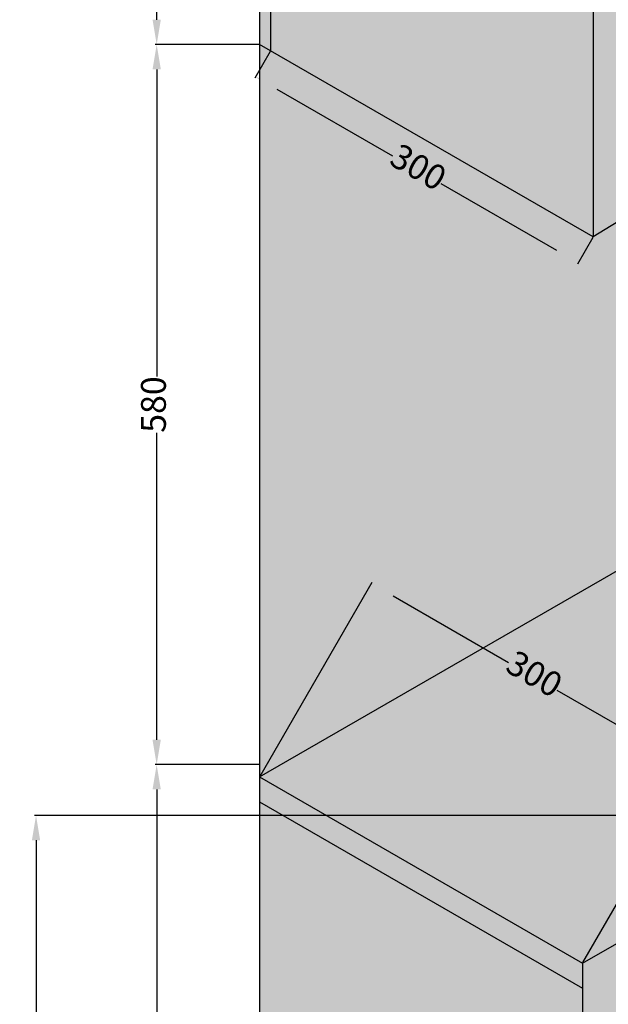
# Model space of a CAD drawing. Units: millimetres. Extents: x 78378 to 86415, y 148682 to 152721.
# Tile 2 of 18: x 78378 to 78851, y 149702 to 150495. Entities that reach past the tile are written whole.
import ezdxf

# ---------------------------------------------------------------- set-up
doc = ezdxf.new("R2010")
doc.units = ezdxf.units.MM
for name, color, linetype, lineweight in [('A-ANNO-DIMS', 2, 'Continuous', 18), ('A-FURN', 4, 'Continuous', 25), ('A-FURN-PATT', 32, 'Continuous', 13)]:
    doc.layers.add(name, color=color, linetype=linetype, lineweight=lineweight)
doc.styles.get("Standard").update_dxf_attribs({"font": 'arial.ttf'})
doc.dimstyles.new('ISO-25', dxfattribs={"dimtxt": 20, "dimasz": 20, "dimexe": 1.25, "dimexo": 0.625, "dimtad": 0, "dimdec": 1, "dimtxsty": 'Standard', "dimcen": 2.5, "dimadec": 0, "dimazin": 0, "dimtfac": 1, "dimtdec": 1, "dimtmove": 0, "dimatfit": 3, "dimfxl": 1, "dimarcsym": 0})

# ---------------------------------------------------------------- blocks, each defined once
blk = doc.blocks.new('*D4')
at = {"layer": 'A-ANNO-DIMS', "color": 0, "lineweight": -2, "transparency": 16777216}
for p, q in [((78570.23, 151205.01), (78486.72, 151205.01)), ((78487.97, 151185.01), (78487.97, 150862.61)), ((78487.97, 150495.01), (78487.97, 150817.4)), ((78570.23, 150475.01), (78486.72, 150475.01))]:
    blk.add_line(p, q, dxfattribs=at)
at = {"layer": 'A-ANNO-DIMS', "color": 0, "transparency": 16777216}
for points in [[(78484.64, 151185.01), (78491.3, 151185.01), (78487.97, 151205.01)], [(78484.64, 150495.01), (78491.3, 150495.01), (78487.97, 150475.01)]]:
    blk.add_solid(points, dxfattribs=at)
at = {"layer": 'Defpoints', "color": 0, "transparency": 16777216}
for p in [(78570.86, 151205.01), (78487.97, 150475.01), (78570.86, 150475.01)]:
    blk.add_point(p, dxfattribs=at)
at = {"layer": 'A-ANNO-DIMS', "color": 0, "transparency": 16777216, "insert": (78487.97, 150840.01), "char_height": 20, "attachment_point": 5, "rotation": 90}
blk.add_mtext('730', dxfattribs=at)
blk = doc.blocks.new('*D5')
at = {"layer": 'A-ANNO-DIMS', "color": 0, "lineweight": -2, "transparency": 16777216}
for p, q in [((78570.23, 150475.01), (78486.72, 150475.01)), ((78487.97, 150455.01), (78487.97, 150207.69)), ((78487.97, 149915.01), (78487.97, 150162.32)), ((78570.23, 149895.01), (78486.72, 149895.01))]:
    blk.add_line(p, q, dxfattribs=at)
at = {"layer": 'A-ANNO-DIMS', "color": 0, "transparency": 16777216}
for points in [[(78484.64, 150455.01), (78491.3, 150455.01), (78487.97, 150475.01)], [(78484.64, 149915.01), (78491.3, 149915.01), (78487.97, 149895.01)]]:
    blk.add_solid(points, dxfattribs=at)
at = {"layer": 'Defpoints', "color": 0, "transparency": 16777216}
for p in [(78570.86, 150475.01), (78487.97, 149895.01), (78570.86, 149895.01)]:
    blk.add_point(p, dxfattribs=at)
at = {"layer": 'A-ANNO-DIMS', "color": 0, "transparency": 16777216, "insert": (78487.97, 150185.01), "char_height": 20, "attachment_point": 5, "rotation": 90}
blk.add_mtext('580', dxfattribs=at)
blk = doc.blocks.new('*D6')
at = {"layer": 'A-ANNO-DIMS', "color": 0, "lineweight": -2, "transparency": 16777216}
for p, q in [((78570.23, 149895.01), (78486.72, 149895.01)), ((78487.97, 149875.01), (78487.97, 149487.71)), ((78487.97, 149055.01), (78487.97, 149442.31)), ((78570.23, 149035.01), (78486.72, 149035.01))]:
    blk.add_line(p, q, dxfattribs=at)
at = {"layer": 'A-ANNO-DIMS', "color": 0, "transparency": 16777216}
for points in [[(78484.64, 149875.01), (78491.3, 149875.01), (78487.97, 149895.01)], [(78484.64, 149055.01), (78491.3, 149055.01), (78487.97, 149035.01)]]:
    blk.add_solid(points, dxfattribs=at)
at = {"layer": 'Defpoints', "color": 0, "transparency": 16777216}
for p in [(78570.86, 149895.01), (78487.97, 149035.01), (78570.86, 149035.01)]:
    blk.add_point(p, dxfattribs=at)
at = {"layer": 'A-ANNO-DIMS', "color": 0, "transparency": 16777216, "insert": (78487.97, 149465.01), "char_height": 20, "attachment_point": 5, "rotation": 90}
blk.add_mtext('860', dxfattribs=at)
blk = doc.blocks.new('*D7')
at = {"layer": 'A-ANNO-DIMS', "color": 0, "lineweight": -2, "transparency": 16777216}
for p, q in [((78579.21, 150469.47), (78566.84, 150448.04)), ((78584.78, 150439.12), (78677.72, 150385.46)), ((78809.95, 150309.12), (78717, 150362.78)), ((78839.02, 150319.47), (78826.64, 150298.04))]:
    blk.add_line(p, q, dxfattribs=at)
at = {"layer": 'A-ANNO-DIMS', "color": 0, "transparency": 16777216}
for points in [[(78586.45, 150442.01), (78583.11, 150436.23), (78567.46, 150449.12)], [(78811.61, 150312.01), (78808.28, 150306.23), (78827.27, 150299.12)]]:
    blk.add_solid(points, dxfattribs=at)
at = {"layer": 'Defpoints', "color": 0, "transparency": 16777216}
for p in [(78579.52, 150470.01), (78567.46, 150449.12), (78839.33, 150320.01)]:
    blk.add_point(p, dxfattribs=at)
at = {"layer": 'A-ANNO-DIMS', "color": 0, "transparency": 16777216, "insert": (78697.36, 150374.12), "char_height": 20, "attachment_point": 5, "rotation": 330}
blk.add_mtext('300', dxfattribs=at)
blk = doc.blocks.new('*D19')
at = {"layer": 'A-ANNO-DIMS', "color": 0, "lineweight": -2, "transparency": 16777216}
for p, q in [((78571.17, 149885.55), (78661.48, 150041.97)), ((78678.18, 150030.89), (78771.12, 149977.23)), ((78903.35, 149900.89), (78810.4, 149954.55)), ((78830.98, 149735.55), (78921.29, 149891.97))]:
    blk.add_line(p, q, dxfattribs=at)
at = {"layer": 'A-ANNO-DIMS', "color": 0, "transparency": 16777216}
for points in [[(78679.85, 150033.78), (78676.51, 150028.01), (78660.86, 150040.89)], [(78905.01, 149903.78), (78901.68, 149898.01), (78920.67, 149890.89)]]:
    blk.add_solid(points, dxfattribs=at)
at = {"layer": 'Defpoints', "color": 0, "transparency": 16777216}
for p in [(78920.67, 149890.89), (78570.86, 149885.01), (78830.67, 149735.01)]:
    blk.add_point(p, dxfattribs=at)
at = {"layer": 'A-ANNO-DIMS', "color": 0, "transparency": 16777216, "insert": (78790.76, 149965.89), "char_height": 20, "attachment_point": 5, "rotation": 330}
blk.add_mtext('300', dxfattribs=at)
blk = doc.blocks.new('*D25')
at = {"layer": 'A-ANNO-DIMS', "color": 0, "lineweight": -2, "transparency": 16777216}
for p, q in [((79360.48, 149854.03), (78389.61, 149854.03)), ((78390.86, 149834.03), (78390.86, 149656.62)), ((78390.86, 149409.86), (78390.86, 149587.28)), ((79360.48, 149389.86), (78389.61, 149389.86))]:
    blk.add_line(p, q, dxfattribs=at)
at = {"layer": 'A-ANNO-DIMS', "color": 0, "transparency": 16777216}
for points in [[(78387.53, 149834.03), (78394.19, 149834.03), (78390.86, 149854.03)], [(78387.53, 149409.86), (78394.19, 149409.86), (78390.86, 149389.86)]]:
    blk.add_solid(points, dxfattribs=at)
at = {"layer": 'Defpoints', "color": 0, "transparency": 16777216}
for p in [(78390.86, 149854.03), (79361.1, 149854.03), (79361.1, 149389.86)]:
    blk.add_point(p, dxfattribs=at)
at = {"layer": 'A-ANNO-DIMS', "color": 0, "transparency": 16777216, "insert": (78390.86, 149621.95), "char_height": 20, "attachment_point": 5, "rotation": 90}
blk.add_mtext('464.2', dxfattribs=at)

msp = doc.modelspace()

# ---------------------------------------------------------------- hatches: boundary and pattern name
at = {"layer": 'A-FURN-PATT'}
h = msp.add_hatch(color=256, dxfattribs=at)
h.dxf.hatch_style = 1
h.paths.add_polyline_path([(78839.3276, 151040.0076), (78579.52, 151190.0076), (78579.52, 150470.0076), (78839.3276, 150320.0076)])
h.paths.add_polyline_path([(79073.1545, 150899.6469, 0.27777969), (79002.2645, 150996.3205, 0.79108393), (78917.9567, 150978.8719, 0.18044832), (78856.6481, 150853.0138), (78856.6481, 150350.6973), (79073.1545, 150484.318)])
h.paths.add_polyline_path([(79073.1545, 151175.0076), (78856.6481, 151050.0076), (78856.6481, 150853.0138, -0.18044832), (78917.9567, 150978.8719, -0.79108393), (79002.2645, 150996.3205, -0.27777969), (79073.1545, 150899.6469)])
h.paths.add_polyline_path([(79341.6224, 151350.0076), (79099.1352, 151490.0076), (78596.8405, 151200.0076), (78839.3276, 151060.0076)])
h.paths.add_polyline_path([(79904.5389, 151675.0076), (79662.0518, 151815.0076), (79099.1352, 151490.0076), (79341.6224, 151350.0076)])
h.paths.add_polyline_path([(80389.5131, 151955.0076), (80389.5131, 152235.0076), (79662.0518, 151815.0076), (79904.5389, 151675.0076)])
h.paths.add_polyline_path([(80389.5131, 151955.0076), (80164.3465, 151825.0076), (80164.3465, 151105.0076), (80614.6797, 151105.0076), (80614.6797, 151825.0076)])
edge = h.paths.add_edge_path(flags=16)
edge.add_spline(control_points=[(80216.308, 151728.251), (80227.1854, 151732.981), (80256.3301, 151745.6544), (80298.41, 151761.9595), (80340.2597, 151805.855), (80391.0771, 151782.0404), (80454.0396, 151805.7581), (80496.5007, 151742.4095), (80543.8218, 151733.4043), (80562.7182, 151729.8083)], knot_values=[0, 0, 0, 0, 35.54374676, 95.23575347, 136.36767513, 200.93298197, 236.72641081, 322.88993498, 380.17027367, 380.17027367, 380.17027367, 380.17027367], degree=3, periodic=0)
edge.add_line((80562.7182, 151729.8083), (80562.7182, 151165.0076))
edge.add_line((80562.7182, 151165.0076), (80216.308, 151165.0076))
edge.add_line((80216.308, 151165.0076), (80216.308, 151728.251))
h.paths.add_polyline_path([(80632.0002, 152095.0076), (80389.5131, 152235.0076), (80389.5131, 151955.0076), (80614.6797, 151825.0076), (80632.0002, 151815.0076)])
h.paths.add_polyline_path([(80867.7794, 151958.8805), (80632.0002, 152095.0076), (80632.0002, 151815.0076), (80632.0002, 151510.0076), (80867.7794, 151373.8805)])
h.paths.add_polyline_path([(80147.026, 151495.8203, 0.18918979), (80063.5671, 151597.7244, 0.78826136), (79979.2691, 151580.5832, 0.16072613), (79904.5389, 151413.5769), (79904.5389, 150955.0076), (80147.026, 151095.0076)])
h.paths.add_polyline_path([(80147.026, 151815.0076), (79904.5389, 151675.0076), (79904.5389, 151413.5769, -0.16072613), (79979.2691, 151580.5832, -0.78826136), (80063.5671, 151597.7244, -0.18918979), (80147.026, 151495.8203)])
h.paths.add_polyline_path([(79887.2184, 151645.0076), (79640.4011, 151502.5076), (79640.4011, 151262.3325, -0.16072613), (79715.1313, 151429.3387, -0.78826136), (79799.4294, 151446.48, -0.21290578), (79887.2184, 151328.7247)])
h.paths.add_polyline_path([(79799.4294, 151446.48, 0.78826136), (79715.1313, 151429.3387, 0.16072613), (79640.4011, 151262.3325), (79640.4011, 150822.5076), (79887.2184, 150965.0076), (79887.2184, 151328.7247, 0.21290578)])
h.paths.add_polyline_path([(79605.7601, 151482.5076), (79358.9429, 151340.0076), (79358.9429, 151100.0701, -0.16072613), (79433.6731, 151267.0764, -0.78826136), (79517.9711, 151284.2176, -0.21290578), (79605.7601, 151166.4623)])
h.paths.add_polyline_path([(79605.7601, 151166.4623, 0.21290578), (79517.9711, 151284.2176, 0.78826136), (79433.6731, 151267.0764, 0.16072613), (79358.9429, 151100.0701), (79358.9429, 150742.9831), (79419.0877, 150694.7323), (79605.7601, 150802.5076)])
edge = h.paths.add_edge_path(flags=0)
edge.add_spline(control_points=[(81152.4356, 151098.7676), (81105.7208, 151145.9466), (81038.6136, 151213.7208), (80882.3866, 151214.1938), (80797.4434, 151311.2997), (80711.8686, 151340.3754), (80681.7691, 151350.6023)], knot_values=[0, 0, 0, 0, 188.233441, 270.4032752, 445.45179201, 540.42858829, 540.42858829, 540.42858829, 540.42858829], degree=3, periodic=0)
edge.add_line((80683.4538, 151350.0269), (80683.4538, 151104.8792))
edge.add_line((80683.4538, 151104.8792), (81152.4356, 150851.399))
edge.add_line((81152.4356, 150851.399), (81152.4356, 151098.7676))
edge = h.paths.add_edge_path(flags=0)
edge.add_spline(control_points=[(80912.9018, 151027.1103), (80892.3742, 151034.1027), (80860.1663, 151045.0739), (80835.5097, 151068.1214), (80826.5679, 151076.4797)], knot_values=[0, 0, 0, 0, 63.98405104, 100.39142428, 100.39142428, 100.39142428, 100.39142428], degree=3, periodic=0)
edge.add_arc((80830.0414, 151081.2992), 5.9407, 100.9277276, 234.2187381, ccw=False)
edge.add_spline(control_points=[(80828.9152, 151087.1322), (80837.857, 151078.7739), (80862.5136, 151055.7263), (80894.7215, 151044.7552), (80915.2491, 151037.7628)], knot_values=[0, 0, 0, 0, 36.40737324, 100.39142428, 100.39142428, 100.39142428, 100.39142428], degree=3, periodic=0)
edge.add_arc((80914.7882, 151032.2795), 5.5026, -107.9540399, 85.195579, ccw=False)
h.paths.add_polyline_path([(81238.218, 151110.0076), (80632.0002, 151460.0076), (80632.0002, 151105.0076), (81238.218, 150755.0076)])
edge = h.paths.add_edge_path(flags=16)
edge.add_line((81152.4356, 150851.399), (80683.4538, 151104.8792))
edge.add_line((80683.4538, 151104.8792), (80683.4538, 151350.0279))
edge.add_spline(control_points=[(80681.7691, 151350.6023), (80711.8686, 151340.3754), (80797.4434, 151311.2997), (80882.3866, 151214.1938), (81038.6136, 151213.7208), (81105.7208, 151145.9466), (81152.4356, 151098.7676)], knot_values=[0, 0, 0, 0, 94.97679628, 270.02531309, 352.19514729, 540.42858829, 540.42858829, 540.42858829, 540.42858829], degree=3, periodic=0)
edge.add_line((81152.4356, 151098.7676), (81152.4356, 150851.399))
edge = h.paths.add_edge_path(flags=0)
edge.add_spline(control_points=[(80912.9018, 151027.1103), (80892.3742, 151034.1027), (80860.1663, 151045.0739), (80835.5097, 151068.1214), (80826.5679, 151076.4797)], knot_values=[0, 0, 0, 0, 63.98405104, 100.39142428, 100.39142428, 100.39142428, 100.39142428], degree=3, periodic=0)
edge.add_arc((80830.0414, 151081.2992), 5.9407, 100.9277276, 234.2187381, ccw=False)
edge.add_spline(control_points=[(80828.9152, 151087.1322), (80837.857, 151078.7739), (80862.5136, 151055.7263), (80894.7215, 151044.7552), (80915.2491, 151037.7628)], knot_values=[0, 0, 0, 0, 36.40737324, 100.39142428, 100.39142428, 100.39142428, 100.39142428], degree=3, periodic=0)
edge.add_arc((80914.7882, 151032.2795), 5.5026, -107.7417882, 85.195579, ccw=False)
h.paths.add_polyline_path([(81498.0256, 151255.0076), (81238.218, 151110.0076), (81238.218, 150755.0076), (81498.0256, 150905.0076)])
edge = h.paths.add_edge_path(flags=16)
edge.add_spline(control_points=[(81152.4356, 151098.7676), (81105.7208, 151145.9466), (81038.6136, 151213.7208), (80882.3866, 151214.1938), (80797.4434, 151311.2997), (80711.8686, 151340.3754), (80681.7691, 151350.6023)], knot_values=[0, 0, 0, 0, 188.233441, 270.4032752, 445.45179201, 540.42858829, 540.42858829, 540.42858829, 540.42858829], degree=3, periodic=0)
edge.add_line((80683.4538, 151350.0279), (80683.4538, 151104.8792))
edge.add_line((80683.4538, 151104.8792), (81152.4356, 150851.399))
edge.add_line((81152.4356, 150851.399), (81152.4356, 151098.7676))
h.paths.add_polyline_path([(81453.9904, 151280.4314), (80867.7794, 151618.8805), (80867.7794, 151373.8805), (81238.218, 151160.0076)])
edge = h.paths.add_edge_path(flags=16)
edge.add_line((81189.2304, 151297.6373), (81114.4166, 151300.2154))
edge.add_arc((81412.0967, 151394.0167), 312.1092, 179.7569303, 197.4900342, ccw=False)
edge.add_ellipse((81154.0183, 151392.0436), major_axis=(-54.0264, 3.6301), ratio=0.22179693, start_angle=0, end_angle=0.3517985, ccw=False)
edge.add_ellipse((81154.0183, 151392.0436), major_axis=(-54.0264, 3.6301), ratio=0.22179693, start_angle=180, end_angle=360, ccw=False)
edge.add_spline(control_points=[(81196.1844, 151321.9476), (81224.9802, 151347.1455), (81266.8846, 151383.8144), (81222.0354, 151387.0304), (81208.0056, 151388.0364)], knot_values=[0, 0, 0, 0, 75.09175173, 109.27580439, 109.27580439, 109.27580439, 109.27580439], degree=3, periodic=0)
edge.add_arc((80751.9112, 151435.6145), 458.5693, 342.4891602, 345.646172, ccw=False)
edge = h.paths.add_edge_path(flags=0)
edge.add_spline(control_points=[(81196.6193, 151323.657), (81197.893, 151324.7717), (81199.1654, 151325.8858), (81209.0233, 151334.5343), (81217.3959, 151341.9835), (81228.0928, 151352.5012), (81231.3883, 151355.9524), (81236.9493, 151362.4395), (81239.214, 151365.4773), (81241.4987, 151369.416), (81242.064, 151370.5542), (81242.9187, 151372.6971), (81243.2076, 151373.7015), (81243.5012, 151375.5539), (81243.5065, 151376.4), (81243.2432, 151377.9407), (81242.9775, 151378.6373), (81242.1402, 151379.937), (81241.5659, 151380.5416), (81240.2039, 151381.533), (81239.4963, 151381.9384), (81237.0619, 151383.0663), (81235.0242, 151383.6999), (81230.352, 151384.7569), (81227.7173, 151385.1826), (81221.9118, 151385.9145), (81218.7193, 151386.2133), (81213.7912, 151386.6115), (81212.1252, 151386.7359), (81209.6196, 151386.9181), (81208.7865, 151386.9779), (81207.9009, 151387.0432)], knot_values=[0.01548744, 0.01548744, 0.01548744, 0.01548744, 3.33787957, 3.33787957, 25.85130624, 25.85130624, 37.52811308, 37.52811308, 49.20491992, 49.20491992, 54.2850938, 54.2850938, 59.36526768, 59.36526768, 64.44544157, 64.44544157, 69.52561545, 69.52561545, 74.60578933, 74.60578933, 78.49366785, 78.49366785, 86.25567095, 86.25567095, 94.01767406, 94.01767406, 102.20226556, 102.20226556, 106.29456131, 106.29456131, 108.32522175, 108.32522175, 108.32522175, 108.32522175], degree=3, periodic=0)
edge = h.paths.add_edge_path(flags=16)
edge.add_arc((81034.1732, 151350.4693), 42.5822, 231.2679035, 306.151846, ccw=False)
edge.add_line((81007.5303, 151317.2517), (81007.5303, 151395.181))
edge.add_ellipse((81033.412, 151394.7791), major_axis=(-25.8816, 0.4538), ratio=0.23894509, start_angle=0, end_angle=0.1147075, ccw=False)
edge.add_ellipse((81033.412, 151394.7791), major_axis=(-25.8816, 0.4538), ratio=0.23894509, start_angle=181.1677709, end_angle=358.9476457, ccw=False)
edge.add_ellipse((81033.412, 151395.7791), major_axis=(-25.8816, 0.4538), ratio=0.23894509, start_angle=180, end_angle=360.1147075, ccw=False)
edge.add_ellipse((81033.412, 151395.7791), major_axis=(-25.8816, 0.4538), ratio=0.23894509, start_angle=178.9476457, end_angle=180, ccw=False)
edge.add_line((81059.2936, 151395.1778), (81059.2936, 151394.3772))
edge.add_ellipse((81033.412, 151394.7791), major_axis=(-25.8816, 0.4538), ratio=0.23894509, start_angle=180, end_angle=180.1147075, ccw=False)
edge.add_ellipse((81033.412, 151394.7791), major_axis=(-25.8816, 0.4538), ratio=0.23894509, start_angle=3.6903098, end_angle=176.4406503, ccw=False)
edge.add_line((81059.2936, 151393.3388), (81059.2936, 151316.086))
h.paths.add_polyline_path([(80951.9355, 151343.9568), (80909.6838, 151362.4635), (80904.0219, 151443.9615, -0.38133308), (80987.2169, 151411.3717)], flags=16)
h = msp.add_hatch(color=256, dxfattribs=at)
h.dxf.hatch_style = 1
h.paths.add_polyline_path([(80389.8136, 150935.1811), (80389.5131, 151105.0076), (80164.3465, 151105.0076), (79904.5389, 150955.0076), (79433.5848, 150683.1022), (79459.4128, 150662.3818), (79243.9048, 150537.9582), (79160.4069, 150518.1674), (78839.3276, 150320.0076), (78579.52, 150470.0076), (78570.8597, 150475.0076), (78570.8597, 150465.0076), (78570.8597, 149885.0076)])
h.paths.add_polyline_path([(80086.4042, 150460.0076), (79826.5966, 150610.0076), (78570.8597, 149885.0076), (78830.6674, 149735.0076)])
h.paths.add_polyline_path([(79540.8001, 150161.0557), (79217.3967, 149974.3386), (78980.9166, 150110.8705), (79304.32, 150297.5875)], flags=16)
h.paths.add_polyline_path([(79506.159, 150161.0557), (79217.3967, 149994.3386), (79015.5576, 150110.8705), (79304.32, 150277.5875)], flags=0)
edge = h.paths.add_edge_path(flags=0)
edge.add_arc((79247.8636, 150177.1541), 137.9799, 256.0025928, 293.5594109)
edge.add_arc((79240.7671, 150078.2605), 68.0855, 336.099104, 387.3696877)
edge.add_ellipse((79258.3074, 150109.4852), major_axis=(-42.6234, -1.6591), ratio=0.16042843, start_angle=0, end_angle=179.0977279, ccw=False)
edge.add_arc((79285.2112, 150074.2509), 77.2096, 155.1233104, 203.6557939)
edge = h.paths.add_edge_path(flags=0)
edge.add_ellipse((79258.6958, 150110.8297), major_axis=(-42.6234, -1.6591), ratio=0.16042843, start_angle=350.6039412, end_angle=356.2289762)
edge.add_line((79219.169, 150111.8937), (79218.3268, 150109.4141))
edge.add_arc((79262.4675, 150032.9602), 88.2813, 112.3931229, 120, ccw=False)
h.paths.add_polyline_path([(79287.0625, 150086.9703, -0.24770206), (79288.1967, 150077.2955, -0.39047651), (79265.4731, 150072.5438, -0.48726153), (79264.079, 150082.3769, 0.39560433)], flags=0)
h.paths.add_polyline_path([(80389.5131, 150935.0076), (79826.5966, 150610.0076), (80086.4042, 150460.0076), (80692.622, 150460.0076), (80952.4296, 150610.0076)])
edge = h.paths.add_edge_path(flags=16)
edge.add_ellipse((80392.4466, 150825.601), major_axis=(-133.0757, 7.722), ratio=0.42449957, start_angle=0, end_angle=360)
edge = h.paths.add_edge_path(flags=0)
edge.add_spline(control_points=[(80269.3541, 150832.7436), (80269.2919, 150831.672), (80269.3503, 150830.5922), (80269.7341, 150828.3361), (80270.0612, 150827.1587), (80271.0461, 150824.6748), (80271.7052, 150823.3692), (80273.4061, 150820.6503), (80274.4481, 150819.2381), (80276.9366, 150816.3509), (80278.3828, 150814.8762), (80282.5858, 150811.0913), (80285.6261, 150808.7701), (80292.6031, 150804.2267), (80296.5388, 150802.0041), (80305.195, 150797.7581), (80309.9151, 150795.7344), (80320.0112, 150791.96), (80325.387, 150790.2092), (80339.2162, 150786.315), (80347.9578, 150784.3563), (80366.0679, 150781.2568), (80375.4359, 150780.1158), (80394.3093, 150778.7158), (80403.8142, 150778.4568), (80422.4656, 150778.8319), (80431.6115, 150779.4662), (80449.0608, 150781.5838), (80457.3636, 150783.0675), (80472.6699, 150786.7766), (80479.6726, 150789.0033), (80490.1894, 150793.2813), (80494.1268, 150795.1967), (80501.0146, 150799.1885), (80503.9632, 150801.2651), (80508.2066, 150804.9015), (80509.73, 150806.4609), (80512.1996, 150809.4942), (80513.1456, 150810.9657), (80514.4291, 150813.5431), (80514.8436, 150814.6688), (80515.3984, 150816.8625), (80515.5405, 150817.9315), (80515.5801, 150820.098), (80515.4773, 150821.1978), (80514.9905, 150823.5062), (80514.6047, 150824.7154), (80513.4854, 150827.2641), (80512.7511, 150828.6027), (80510.8872, 150831.3809), (80509.7578, 150832.8196), (80507.0873, 150835.7513), (80505.5466, 150837.2439), (80501.0624, 150841.0944), (80497.8199, 150843.4576), (80490.4174, 150848.062), (80486.2582, 150850.3037), (80477.1448, 150854.5643), (80472.1909, 150856.5835), (80461.6275, 150860.3245), (80456.0182, 150862.0465), (80441.7332, 150865.8127), (80432.7885, 150867.6675), (80414.3391, 150870.5317), (80404.8349, 150871.5411), (80385.7707, 150872.6572), (80376.2113, 150872.764), (80357.5444, 150872.0728), (80348.4375, 150871.2748), (80331.1682, 150868.83), (80323.0064, 150867.1827), (80309.472, 150863.5363), (80303.8628, 150861.6593), (80293.8018, 150857.5401), (80289.3512, 150855.2969), (80282.7757, 150851.2345), (80280.3473, 150849.4579), (80276.2606, 150845.9127), (80274.604, 150844.1458), (80272.3157, 150841.1243), (80271.5358, 150839.8454), (80270.3496, 150837.3879), (80269.9417, 150836.2101), (80269.5065, 150834.2815), (80269.3988, 150833.5143), (80269.3541, 150832.7436)], knot_values=[0, 0, 0, 0, 0.09750046, 0.09750046, 0.19500092, 0.19500092, 0.29250138, 0.29250138, 0.39000184, 0.39000184, 0.4875023, 0.4875023, 0.63880322, 0.63880322, 0.79010415, 0.79010415, 0.94140507, 0.94140507, 1.092706, 1.092706, 1.3128171, 1.3128171, 1.5329282, 1.5329282, 1.7530393, 1.7530393, 1.97315041, 1.97315041, 2.19326151, 2.19326151, 2.41337261, 2.41337261, 2.56986063, 2.56986063, 2.72634866, 2.72634866, 2.84418658, 2.84418658, 2.96202451, 2.96202451, 3.06023388, 3.06023388, 3.15844325, 3.15844325, 3.25665261, 3.25665261, 3.35486198, 3.35486198, 3.45307135, 3.45307135, 3.55128072, 3.55128072, 3.64949009, 3.64949009, 3.80392773, 3.80392773, 3.95836537, 3.95836537, 4.11280301, 4.11280301, 4.26724064, 4.26724064, 4.48920349, 4.48920349, 4.71116635, 4.71116635, 4.9331292, 4.9331292, 5.15509205, 5.15509205, 5.3770549, 5.3770549, 5.55785361, 5.55785361, 5.73865232, 5.73865232, 5.87239556, 5.87239556, 6.00613879, 6.00613879, 6.109605, 6.109605, 6.2130712, 6.2130712, 6.28318531, 6.28318531, 6.28318531, 6.28318531], degree=3, periodic=0)
edge = h.paths.add_edge_path(flags=0)
edge.add_ellipse((80392.4466, 150825.601), major_axis=(-101.8398, 3.3923), ratio=0.40349248, start_angle=0, end_angle=360)
edge = h.paths.add_edge_path(flags=0)
edge.add_ellipse((80391.1657, 150858.3746), major_axis=(9.0882, -0.6733), ratio=0.35135413, start_angle=0, end_angle=360)
h.paths.add_polyline_path([(80952.4296, 150610.0076), (80692.622, 150460.0076), (81361.2342, 150073.9842), (81649.9628, 150052.7286), (81766.4935, 150120.0076), (81766.4935, 150140.0076), (81564.9025, 150256.3963), (81564.8884, 150096.1963), (81538.9076, 150111.1963), (81538.9217, 150271.3963)])
h.paths.add_polyline_path([(81539.0357, 151571.3305), (80867.7794, 151958.8805), (80867.7794, 151618.8805), (81498.0256, 151255.0076), (81498.0256, 150905.0076), (81238.218, 150755.0076), (81538.9488, 150581.3806)])
h.paths.add_polyline_path([(81766.4935, 151440.0076), (81565.0164, 151556.3305), (81564.9296, 150566.3806), (81766.4935, 150450.0076)])
edge = h.paths.add_edge_path()
edge.add_line((81564.9296, 150566.3806), (81564.9137, 150384.6289))
edge.add_ellipse((81552.1304, 150358.5718), major_axis=(52.6272, 3.506), ratio=0.49589905, start_angle=367.5169757, end_angle=420.0564686, ccw=False)
edge.add_ellipse((81552.1304, 150358.5718), major_axis=(52.6272, 3.506), ratio=0.49589905, start_angle=351.729742, end_angle=367.5169757, ccw=False)
edge.add_ellipse((81552.1304, 150345.5016), major_axis=(52.6272, 3.506), ratio=0.49589905, start_angle=352.5116949, end_angle=366.3006092, ccw=False)
edge.add_line((81603.4463, 150342.2039), (81603.5064, 150340.4475))
edge.add_ellipse((81552.1304, 150332.128), major_axis=(52.6272, 3.506), ratio=0.49589905, start_angle=353.6729654, end_angle=365.3867997, ccw=False)
edge.add_ellipse((81552.1304, 150332.128), major_axis=(52.6272, 3.506), ratio=0.49589905, start_angle=350.9388331, end_angle=353.6729654)
edge.add_line((81603.8688, 150329.855), (81604.0442, 150324.7302))
edge.add_ellipse((81552.1304, 150317.7418), major_axis=(52.6272, 3.506), ratio=0.49589905, start_angle=355.2176746, end_angle=363.8553364, ccw=False)
edge.add_ellipse((81552.1304, 150317.7418), major_axis=(52.6272, 3.506), ratio=0.49589905, start_angle=341.3250873, end_angle=355.2176746, ccw=False)
edge.add_ellipse((81552.1304, 150317.7418), major_axis=(52.6272, 3.506), ratio=0.49589905, start_angle=293.4661701, end_angle=341.3250873, ccw=False)
edge.add_line((81564.9057, 150292.9664), (81564.9025, 150256.3963))
edge.add_line((81564.9025, 150256.3963), (81766.4935, 150140.0076))
edge.add_line((81766.4935, 150140.0076), (81766.4935, 150450.0076))
edge.add_line((81766.4935, 150450.0076), (81564.9296, 150566.3806))
h.paths.add_polyline_path([(81525.5713, 150321.598), (81526.5985, 150321.3069), (81528.6771, 150320.947)])
h.paths.add_polyline_path([(81512.7903, 150326.1129), (81514.5058, 150325.3887), (81512.538, 150326.2678)])
h.paths.add_polyline_path([(81533.2148, 150320.1615), (81534.6952, 150319.9052), (81536.5995, 150319.7557)])
h.paths.add_polyline_path([(81518.622, 150323.6513), (81519.227, 150323.3959), (81521.289, 150322.8116)])
h.paths.add_polyline_path([(81501.2183, 150336.2599), (81500.3543, 150338.1339), (81499.7815, 150340.0494), (81499.5032, 150341.9955), (81499.5032, 150343.7257), (81499.7584, 150345.5905), (81500.2766, 150347.4549), (81501.0551, 150349.3095), (81501.0967, 150349.3937), (81501.1389, 150349.4778), (81500.9978, 150349.7496), (81500.8628, 150350.0225), (81499.5032, 150355.0658), (81499.9591, 150359.5002), (81501.8982, 150363.9083), (81505.2653, 150368.1646), (81509.9647, 150372.1482), (81515.8627, 150375.7459), (81522.7918, 150378.8553), (81530.555, 150381.3882), (81538.9315, 150383.2724), (81538.9488, 150581.3806), (80632.0002, 151105.0076), (80389.5131, 151105.0076), (80389.8142, 150934.8338), (80952.4296, 150610.0076), (81538.9217, 150271.3963), (81538.9234, 150291.7194), (81538.8752, 150291.721), (81530.1915, 150292.8239), (81522.1802, 150294.6904), (81515.0866, 150297.2633), (81509.8635, 150299.9959), (81505.6084, 150303.1351), (81502.419, 150306.6088), (81500.3683, 150310.3375), (81499.5032, 150314.2358), (81499.5032, 150315.9659), (81499.8206, 150318.1159), (81500.487, 150320.2634), (81501.4979, 150322.3941), (81500.487, 150324.4233), (81499.8206, 150326.5039), (81499.5032, 150328.622), (81499.5032, 150330.3521), (81499.7815, 150332.3262), (81500.3543, 150334.2992)])
h = msp.add_hatch(color=256, dxfattribs=at)
h.dxf.hatch_style = 1
h.paths.add_polyline_path([(79090.475, 151205.0076), (78839.3276, 151060.0076), (78839.3276, 150320.0076), (79090.475, 150475.0076)])
h.paths.add_polyline_path([(79073.1545, 151175.0076), (79073.1545, 150899.6469, -0.04544363), (79073.1545, 150878.5653), (79073.1545, 150484.318), (78856.6481, 150350.6973), (78856.6481, 150814.5249, -0.04815716), (78856.6481, 150853.0138), (78856.6481, 151050.0076)], flags=16)
h.paths.add_polyline_path([(79358.9429, 151340.0076), (79605.7601, 151482.5076), (79605.7601, 150802.5076), (79419.0877, 150694.7323), (79433.5848, 150683.1022), (79623.0806, 150792.5076), (79623.0806, 151512.5076), (79341.6224, 151350.0076), (79341.6224, 150756.8784), (79358.9429, 150742.9831)])
h.paths.add_polyline_path([(79341.6224, 151350.0076), (79090.475, 151205.0076), (79090.475, 150475.0076), (79160.4069, 150518.1674), (79107.7955, 150505.6973), (79107.7955, 151195.0076), (79109.5275, 151196.0076), (79324.3018, 151320.0076), (79324.3018, 150770.7736), (79341.6224, 150756.8784)])
h.paths.add_polyline_path([(79887.2184, 151645.0076), (79887.2184, 151665.0076), (79623.0806, 151512.5076), (79623.0806, 150792.5076), (79887.2184, 150945.0076), (79887.2184, 150965.0076), (79640.4011, 150822.5076), (79640.4011, 151502.5076)])
h.paths.add_polyline_path([(79904.5389, 151655.0076), (79887.2184, 151645.0076), (79887.2184, 150965.0076), (79904.5389, 150975.0076)])
h.paths.add_polyline_path([(80164.3465, 151825.0076), (80147.026, 151815.0076), (80147.026, 151095.0076), (80164.3465, 151105.0076)])
h.paths.add_polyline_path([(80632.0002, 151510.0076), (80632.0002, 151490.0076), (81238.218, 151140.0076), (81471.6045, 151270.2619), (81453.9904, 151280.4314), (81238.218, 151160.0076)])
h.paths.add_polyline_path([(80632.0002, 151490.0076), (80632.0002, 151470.0076), (81238.218, 151120.0076), (81489.2186, 151260.0924), (81471.6045, 151270.2619), (81238.218, 151140.0076)])
h.paths.add_polyline_path([(80632.0002, 151460.0076), (80632.0002, 151105.0076), (81238.218, 150755.0076), (81238.218, 151110.0076)])
edge = h.paths.add_edge_path(flags=16)
edge.add_spline(control_points=[(80681.7691, 151350.6023), (80711.8686, 151340.3754), (80797.4434, 151311.2997), (80882.3866, 151214.1938), (81038.6136, 151213.7208), (81105.7208, 151145.9466), (81152.4356, 151098.7676)], knot_values=[0, 0, 0, 0, 94.97679628, 270.02531309, 352.19514729, 540.42858829, 540.42858829, 540.42858829, 540.42858829], degree=3, periodic=0)
edge.add_line((81152.4356, 151098.7676), (81152.4356, 150851.399))
edge.add_line((81152.4356, 150851.399), (80683.4538, 151104.8792))
edge.add_line((80683.4538, 151104.8792), (80683.4538, 151350.027))
edge = h.paths.add_edge_path(flags=0)
edge.add_spline(control_points=[(80828.9152, 151087.1322), (80837.857, 151078.7739), (80862.5136, 151055.7263), (80894.7215, 151044.7552), (80915.2491, 151037.7628)], knot_values=[0, 0, 0, 0, 36.40737324, 100.39142428, 100.39142428, 100.39142428, 100.39142428], degree=3, periodic=0)
edge.add_arc((80914.7882, 151032.2795), 5.5026, -107.9540399, 85.195579, ccw=False)
edge.add_spline(control_points=[(80912.9018, 151027.1103), (80892.3742, 151034.1027), (80860.1663, 151045.0739), (80835.5097, 151068.1214), (80826.5679, 151076.4797)], knot_values=[0, 0, 0, 0, 63.98405104, 100.39142428, 100.39142428, 100.39142428, 100.39142428], degree=3, periodic=0)
edge.add_arc((80830.0414, 151081.2992), 5.9407, 100.9277276, 234.2187381, ccw=False)
h.paths.add_polyline_path([(80632.0002, 151815.0076), (80614.6797, 151825.0076), (80614.6797, 151105.0076), (80632.0002, 151105.0076)])
h.paths.add_polyline_path([(81498.0256, 151255.0076), (81489.2186, 151260.0924), (81238.218, 151120.0076), (80632.0002, 151470.0076), (80632.0002, 151460.0076), (81238.218, 151110.0076)])
h.paths.add_polyline_path([(78596.8405, 151200.0076), (78579.52, 151190.0076), (78839.3276, 151040.0076), (78839.3276, 151060.0076)])
h.paths.add_polyline_path([(78596.8405, 151200.0076), (78579.52, 151210.0076), (78579.52, 151190.0076)])
h.paths.add_polyline_path([(78579.52, 151210.0076), (78570.8597, 151205.0076), (78570.8597, 150475.0076), (78579.52, 150470.0076)])
h = msp.add_hatch(color=256, dxfattribs=at)
h.dxf.hatch_style = 1
h.paths.add_polyline_path([(78830.6674, 149715.0076), (78570.8597, 149865.0076), (78570.8597, 149055.0076), (78830.6674, 148905.0076)])
h.paths.add_polyline_path([(79257.8556, 149981.6449), (78830.6674, 149735.0076), (78830.6674, 148905.0076), (79257.8556, 149151.6449)])
h.paths.add_polyline_path([(79116.9453, 149653.5787, -0.33999439), (79231.8748, 149531.6449), (79231.8748, 149166.6449), (78856.6481, 148950.0076), (78856.6481, 149398.1143, -0.25342364), (78959.4208, 149588.1766, -0.77714453)], flags=16)
h.paths.add_polyline_path([(79231.8748, 149531.6449, 0.33999439), (79116.9453, 149653.5787, 0.77714453), (78959.4208, 149588.1766, 0.25342364), (78856.6481, 149398.1143), (78856.6481, 148950.0076), (79231.8748, 149166.6449)], flags=0)
h = msp.add_hatch(color=256, dxfattribs=at)
h.dxf.hatch_style = 1
h.paths.add_polyline_path([(78570.8597, 149885.0076), (78570.8597, 149865.0076), (78830.6674, 149715.0076), (78830.6674, 149735.0076)])

# ---------------------------------------------------------------- linework, layer by layer
at = {"layer": 'A-FURN'}
for p, q in [((78570.8597, 151205.0076), (78570.8597, 150465.0076)), ((78579.52, 151210.0076), (78579.52, 150470.0076)), ((78839.3276, 151060.0076), (78839.3276, 150320.0076)), ((78570.8597, 149885.0076), (80389.5131, 150935.0076)), ((79160.4069, 150518.1674), (78839.3276, 150320.0076)), ((78579.52, 150470.0076), (78570.8597, 150475.0076)), ((78839.3276, 150320.0076), (78579.52, 150470.0076)), ((78570.8597, 150465.0076), (78570.8597, 149885.0076)), ((78830.6674, 149735.0076), (80086.4042, 150460.0076)), ((78570.8597, 149885.0076), (78570.8597, 149025.0076)), ((78570.8597, 149885.0076), (78830.6674, 149735.0076)), ((78570.8597, 149865.0076), (78830.6674, 149715.0076)), ((78830.6674, 149735.0076), (78830.6674, 148875.0076))]:
    msp.add_line(p, q, dxfattribs=at)

# ---------------------------------------------------------------- dimensions: what is measured, and where the dimension line sits
at = {"layer": 'A-ANNO-DIMS'}
for p1, p2, distance, picture, middle in [((78570.8597, 151205.0076), (78570.8597, 150475.0076), -82.8905, '*D4', (78487.9692, 150840.0076)), ((78570.8597, 150475.0076), (78570.8597, 149895.0076), -82.8905, '*D5', (78487.9692, 150185.0076)), ((78839.3276, 150320.0076), (78579.52, 150470.0076), 24.1188, '*D7', (78697.3644, 150374.1202)), ((78570.8597, 149895.0076), (78570.8597, 149035.0076), -82.8905, '*D6', (78487.9692, 149465.0076))]:
    dim = msp.add_aligned_dim(p1=p1, p2=p2, distance=distance, dimstyle='ISO-25', override={"dimclrd": 0, "dimclre": 0, "dimclrt": 0}, dxfattribs=at)
    dim.commit()
    dim.dimension.update_dxf_attribs({"geometry": picture, "text_midpoint": middle})
for base, p1, p2, angle, override, picture, middle in [((78920.6674, 149890.8922), (78570.8597, 149885.0076), (78830.6674, 149735.0076), 330, {"dimdec": 0, "dimlfac": 1, "dimrnd": 0, "dimzin": 0, "dimdsep": 46, "dimlunit": 2}, '*D19', (78790.7636, 149965.8922)), ((78390.8597, 149854.0252), (79361.1019, 149389.8649), (79361.1019, 149854.0252), 90, {"dimdec": 1, "dimlfac": 1, "dimrnd": 0, "dimzin": 0, "dimdsep": 46, "dimlunit": 2}, '*D25', (78390.8597, 149621.945))]:
    dim = msp.add_linear_dim(base=base, p1=p1, p2=p2, angle=angle, dimstyle='ISO-25', override=override, dxfattribs=at)
    dim.commit()
    dim.dimension.update_dxf_attribs({"geometry": picture, "text_midpoint": middle})

doc.saveas('drawing.dxf')
